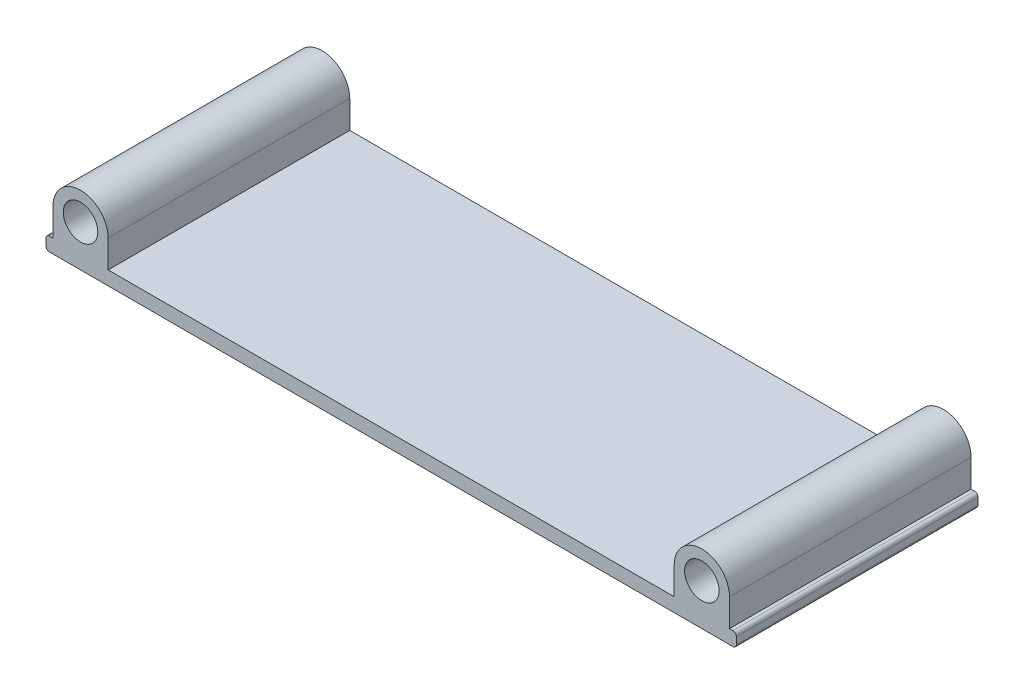
ISO-10303-21;
HEADER;
FILE_DESCRIPTION(('STEP AP214'),'2;1');
FILE_NAME('part.step','',(''),(''),'','','');
FILE_SCHEMA(('AUTOMOTIVE_DESIGN { 1 0 10303 214 1 1 1 1 }'));
ENDSEC;
DATA;
#1=APPLICATION_CONTEXT('core data for automotive mechanical design processes');
#2=APPLICATION_PROTOCOL_DEFINITION('international standard','automotive_design',2000,#1);
#3=PRODUCT_CONTEXT('',#1,'mechanical');
#4=PRODUCT('Part','Part','',(#3));
#5=PRODUCT_RELATED_PRODUCT_CATEGORY('part','',(#4));
#6=PRODUCT_DEFINITION_FORMATION('','',#4);
#7=PRODUCT_DEFINITION_CONTEXT('part definition',#1,'design');
#8=PRODUCT_DEFINITION('design','',#6,#7);
#9=PRODUCT_DEFINITION_SHAPE('','',#8);
#10=(LENGTH_UNIT() NAMED_UNIT(*) SI_UNIT(.MILLI.,.METRE.));
#11=(NAMED_UNIT(*) PLANE_ANGLE_UNIT() SI_UNIT($,.RADIAN.));
#12=(NAMED_UNIT(*) SI_UNIT($,.STERADIAN.) SOLID_ANGLE_UNIT());
#13=UNCERTAINTY_MEASURE_WITH_UNIT(LENGTH_MEASURE(1.E-05),#10,'distance_accuracy_value','');
#14=(GEOMETRIC_REPRESENTATION_CONTEXT(3) GLOBAL_UNCERTAINTY_ASSIGNED_CONTEXT((#13)) GLOBAL_UNIT_ASSIGNED_CONTEXT((#10,
#11,#12)) REPRESENTATION_CONTEXT('',''));
#15=CARTESIAN_POINT('',(0.,0.,0.));
#16=DIRECTION('',(0.,0.,1.));
#17=DIRECTION('',(1.,0.,0.));
#18=AXIS2_PLACEMENT_3D('',#15,#16,#17);
#19=CARTESIAN_POINT('',(49.,0.,17.5));
#20=DIRECTION('',(-1.,0.,0.));
#21=DIRECTION('',(0.,0.,1.));
#22=AXIS2_PLACEMENT_3D('',#19,#20,#21);
#23=PLANE('',#22);
#24=DIRECTION('',(0.,1.,0.));
#25=VECTOR('',#24,1.);
#26=CARTESIAN_POINT('',(49.,0.,-17.5));
#27=LINE('',#26,#25);
#28=CARTESIAN_POINT('',(49.,1.,-17.5));
#29=VERTEX_POINT('',#28);
#30=CARTESIAN_POINT('',(49.,5.,-17.5));
#31=VERTEX_POINT('',#30);
#32=EDGE_CURVE('E176',#29,#31,#27,.T.);
#33=ORIENTED_EDGE('',*,*,#32,.T.);
#34=DIRECTION('',(0.,0.,-1.));
#35=VECTOR('',#34,1.);
#36=CARTESIAN_POINT('',(49.,5.,17.5));
#37=LINE('',#36,#35);
#38=CARTESIAN_POINT('',(49.,5.,17.5));
#39=VERTEX_POINT('',#38);
#40=EDGE_CURVE('E161',#39,#31,#37,.T.);
#41=ORIENTED_EDGE('',*,*,#40,.F.);
#42=DIRECTION('',(0.,1.,0.));
#43=VECTOR('',#42,1.);
#44=CARTESIAN_POINT('',(49.,0.,17.5));
#45=LINE('',#44,#43);
#46=CARTESIAN_POINT('',(49.,1.,17.5));
#47=VERTEX_POINT('',#46);
#48=EDGE_CURVE('E170',#47,#39,#45,.T.);
#49=ORIENTED_EDGE('',*,*,#48,.F.);
#50=DIRECTION('',(0.,0.,-1.));
#51=VECTOR('',#50,1.);
#52=CARTESIAN_POINT('',(49.,1.,17.5));
#53=LINE('',#52,#51);
#54=EDGE_CURVE('E245',#47,#29,#53,.T.);
#55=ORIENTED_EDGE('',*,*,#54,.T.);
#56=EDGE_LOOP('',(#33,#41,#49,#55));
#57=FACE_BOUND('',#56,.T.);
#58=ADVANCED_FACE('F41',(#57),#23,.F.);
#59=CARTESIAN_POINT('',(45.,5.,17.5));
#60=DIRECTION('',(0.,0.,-1.));
#61=DIRECTION('',(-1.,0.,0.));
#62=AXIS2_PLACEMENT_3D('',#59,#60,#61);
#63=CYLINDRICAL_SURFACE('',#62,4.);
#64=CARTESIAN_POINT('',(45.,5.,-17.5));
#65=DIRECTION('',(0.,0.,1.));
#66=DIRECTION('',(1.,0.,0.));
#67=AXIS2_PLACEMENT_3D('',#64,#65,#66);
#68=CIRCLE('',#67,4.);
#69=CARTESIAN_POINT('',(41.,5.,-17.5));
#70=VERTEX_POINT('',#69);
#71=EDGE_CURVE('E267',#31,#70,#68,.T.);
#72=ORIENTED_EDGE('',*,*,#71,.T.);
#73=DIRECTION('',(0.,0.,-1.));
#74=VECTOR('',#73,1.);
#75=CARTESIAN_POINT('',(41.,5.,17.5));
#76=LINE('',#75,#74);
#77=CARTESIAN_POINT('',(41.,5.,17.5));
#78=VERTEX_POINT('',#77);
#79=EDGE_CURVE('E162',#78,#70,#76,.T.);
#80=ORIENTED_EDGE('',*,*,#79,.F.);
#81=CARTESIAN_POINT('',(45.,5.,17.5));
#82=DIRECTION('',(0.,0.,1.));
#83=DIRECTION('',(1.,0.,0.));
#84=AXIS2_PLACEMENT_3D('',#81,#82,#83);
#85=CIRCLE('',#84,4.);
#86=EDGE_CURVE('E156',#39,#78,#85,.T.);
#87=ORIENTED_EDGE('',*,*,#86,.F.);
#88=ORIENTED_EDGE('',*,*,#40,.T.);
#89=EDGE_LOOP('',(#72,#80,#87,#88));
#90=FACE_BOUND('',#89,.T.);
#91=ADVANCED_FACE('F157',(#90),#63,.T.);
#92=CARTESIAN_POINT('',(41.,0.,17.5));
#93=DIRECTION('',(-1.,0.,0.));
#94=DIRECTION('',(0.,0.,1.));
#95=AXIS2_PLACEMENT_3D('',#92,#93,#94);
#96=PLANE('',#95);
#97=DIRECTION('',(0.,1.,0.));
#98=VECTOR('',#97,1.);
#99=CARTESIAN_POINT('',(41.,0.,-17.5));
#100=LINE('',#99,#98);
#101=CARTESIAN_POINT('',(41.,1.,-17.5));
#102=VERTEX_POINT('',#101);
#103=EDGE_CURVE('E270',#102,#70,#100,.T.);
#104=ORIENTED_EDGE('',*,*,#103,.F.);
#105=DIRECTION('',(0.,0.,-1.));
#106=VECTOR('',#105,1.);
#107=CARTESIAN_POINT('',(41.,1.,17.5));
#108=LINE('',#107,#106);
#109=CARTESIAN_POINT('',(41.,1.,17.5));
#110=VERTEX_POINT('',#109);
#111=EDGE_CURVE('E181',#110,#102,#108,.T.);
#112=ORIENTED_EDGE('',*,*,#111,.F.);
#113=DIRECTION('',(0.,1.,0.));
#114=VECTOR('',#113,1.);
#115=CARTESIAN_POINT('',(41.,0.,17.5));
#116=LINE('',#115,#114);
#117=EDGE_CURVE('E167',#110,#78,#116,.T.);
#118=ORIENTED_EDGE('',*,*,#117,.T.);
#119=ORIENTED_EDGE('',*,*,#79,.T.);
#120=EDGE_LOOP('',(#104,#112,#118,#119));
#121=FACE_BOUND('',#120,.T.);
#122=ADVANCED_FACE('F268',(#121),#96,.T.);
#123=CARTESIAN_POINT('',(0.,1.,17.5));
#124=DIRECTION('',(0.,1.,0.));
#125=DIRECTION('',(0.,0.,1.));
#126=AXIS2_PLACEMENT_3D('',#123,#124,#125);
#127=PLANE('',#126);
#128=DIRECTION('',(1.,0.,0.));
#129=VECTOR('',#128,1.);
#130=CARTESIAN_POINT('',(0.,1.,-17.5));
#131=LINE('',#130,#129);
#132=CARTESIAN_POINT('',(-41.,1.,-17.5));
#133=VERTEX_POINT('',#132);
#134=EDGE_CURVE('E265',#133,#102,#131,.T.);
#135=ORIENTED_EDGE('',*,*,#134,.F.);
#136=DIRECTION('',(0.,0.,-1.));
#137=VECTOR('',#136,1.);
#138=CARTESIAN_POINT('',(-41.,1.,17.5));
#139=LINE('',#138,#137);
#140=CARTESIAN_POINT('',(-41.,1.,17.5));
#141=VERTEX_POINT('',#140);
#142=EDGE_CURVE('E254',#141,#133,#139,.T.);
#143=ORIENTED_EDGE('',*,*,#142,.F.);
#144=DIRECTION('',(1.,0.,0.));
#145=VECTOR('',#144,1.);
#146=CARTESIAN_POINT('',(0.,1.,17.5));
#147=LINE('',#146,#145);
#148=EDGE_CURVE('E262',#141,#110,#147,.T.);
#149=ORIENTED_EDGE('',*,*,#148,.T.);
#150=ORIENTED_EDGE('',*,*,#111,.T.);
#151=EDGE_LOOP('',(#135,#143,#149,#150));
#152=FACE_BOUND('',#151,.T.);
#153=ADVANCED_FACE('F257',(#152),#127,.T.);
#154=CARTESIAN_POINT('',(-41.,0.,17.5));
#155=DIRECTION('',(-1.,0.,0.));
#156=DIRECTION('',(0.,0.,1.));
#157=AXIS2_PLACEMENT_3D('',#154,#155,#156);
#158=PLANE('',#157);
#159=DIRECTION('',(0.,1.,0.));
#160=VECTOR('',#159,1.);
#161=CARTESIAN_POINT('',(-41.,0.,-17.5));
#162=LINE('',#161,#160);
#163=CARTESIAN_POINT('',(-41.,5.,-17.5));
#164=VERTEX_POINT('',#163);
#165=EDGE_CURVE('E272',#133,#164,#162,.T.);
#166=ORIENTED_EDGE('',*,*,#165,.T.);
#167=DIRECTION('',(0.,0.,-1.));
#168=VECTOR('',#167,1.);
#169=CARTESIAN_POINT('',(-41.,5.,17.5));
#170=LINE('',#169,#168);
#171=CARTESIAN_POINT('',(-41.,5.,17.5));
#172=VERTEX_POINT('',#171);
#173=EDGE_CURVE('E252',#172,#164,#170,.T.);
#174=ORIENTED_EDGE('',*,*,#173,.F.);
#175=DIRECTION('',(0.,1.,0.));
#176=VECTOR('',#175,1.);
#177=CARTESIAN_POINT('',(-41.,0.,17.5));
#178=LINE('',#177,#176);
#179=EDGE_CURVE('E299',#141,#172,#178,.T.);
#180=ORIENTED_EDGE('',*,*,#179,.F.);
#181=ORIENTED_EDGE('',*,*,#142,.T.);
#182=EDGE_LOOP('',(#166,#174,#180,#181));
#183=FACE_BOUND('',#182,.T.);
#184=ADVANCED_FACE('F298',(#183),#158,.F.);
#185=CARTESIAN_POINT('',(-45.,5.,17.5));
#186=DIRECTION('',(0.,0.,-1.));
#187=DIRECTION('',(-1.,0.,0.));
#188=AXIS2_PLACEMENT_3D('',#185,#186,#187);
#189=CYLINDRICAL_SURFACE('',#188,4.);
#190=CARTESIAN_POINT('',(-45.,5.,-17.5));
#191=DIRECTION('',(0.,0.,1.));
#192=DIRECTION('',(1.,0.,0.));
#193=AXIS2_PLACEMENT_3D('',#190,#191,#192);
#194=CIRCLE('',#193,4.);
#195=CARTESIAN_POINT('',(-49.,5.,-17.5));
#196=VERTEX_POINT('',#195);
#197=EDGE_CURVE('E274',#164,#196,#194,.T.);
#198=ORIENTED_EDGE('',*,*,#197,.T.);
#199=DIRECTION('',(0.,0.,-1.));
#200=VECTOR('',#199,1.);
#201=CARTESIAN_POINT('',(-49.,5.,17.5));
#202=LINE('',#201,#200);
#203=CARTESIAN_POINT('',(-49.,5.,17.5));
#204=VERTEX_POINT('',#203);
#205=EDGE_CURVE('E249',#204,#196,#202,.T.);
#206=ORIENTED_EDGE('',*,*,#205,.F.);
#207=CARTESIAN_POINT('',(-45.,5.,17.5));
#208=DIRECTION('',(0.,0.,1.));
#209=DIRECTION('',(1.,0.,0.));
#210=AXIS2_PLACEMENT_3D('',#207,#208,#209);
#211=CIRCLE('',#210,4.);
#212=EDGE_CURVE('E291',#172,#204,#211,.T.);
#213=ORIENTED_EDGE('',*,*,#212,.F.);
#214=ORIENTED_EDGE('',*,*,#173,.T.);
#215=EDGE_LOOP('',(#198,#206,#213,#214));
#216=FACE_BOUND('',#215,.T.);
#217=ADVANCED_FACE('F292',(#216),#189,.T.);
#218=CARTESIAN_POINT('',(-49.,0.,17.5));
#219=DIRECTION('',(-1.,0.,0.));
#220=DIRECTION('',(0.,0.,1.));
#221=AXIS2_PLACEMENT_3D('',#218,#219,#220);
#222=PLANE('',#221);
#223=DIRECTION('',(0.,1.,0.));
#224=VECTOR('',#223,1.);
#225=CARTESIAN_POINT('',(-49.,0.,-17.5));
#226=LINE('',#225,#224);
#227=CARTESIAN_POINT('',(-49.,1.,-17.5));
#228=VERTEX_POINT('',#227);
#229=EDGE_CURVE('E231',#228,#196,#226,.T.);
#230=ORIENTED_EDGE('',*,*,#229,.F.);
#231=DIRECTION('',(0.,0.,-1.));
#232=VECTOR('',#231,1.);
#233=CARTESIAN_POINT('',(-49.,1.,17.5));
#234=LINE('',#233,#232);
#235=CARTESIAN_POINT('',(-49.,1.,17.5));
#236=VERTEX_POINT('',#235);
#237=EDGE_CURVE('E248',#236,#228,#234,.T.);
#238=ORIENTED_EDGE('',*,*,#237,.F.);
#239=DIRECTION('',(0.,1.,0.));
#240=VECTOR('',#239,1.);
#241=CARTESIAN_POINT('',(-49.,0.,17.5));
#242=LINE('',#241,#240);
#243=EDGE_CURVE('E286',#236,#204,#242,.T.);
#244=ORIENTED_EDGE('',*,*,#243,.T.);
#245=ORIENTED_EDGE('',*,*,#205,.T.);
#246=EDGE_LOOP('',(#230,#238,#244,#245));
#247=FACE_BOUND('',#246,.T.);
#248=ADVANCED_FACE('F285',(#247),#222,.T.);
#249=CARTESIAN_POINT('',(0.,1.,17.5));
#250=DIRECTION('',(0.,1.,0.));
#251=DIRECTION('',(0.,0.,1.));
#252=AXIS2_PLACEMENT_3D('',#249,#250,#251);
#253=PLANE('',#252);
#254=DIRECTION('',(1.,0.,0.));
#255=VECTOR('',#254,1.);
#256=CARTESIAN_POINT('',(0.,1.,-17.5));
#257=LINE('',#256,#255);
#258=CARTESIAN_POINT('',(-49.5,1.,-17.5));
#259=VERTEX_POINT('',#258);
#260=EDGE_CURVE('E227',#259,#228,#257,.T.);
#261=ORIENTED_EDGE('',*,*,#260,.F.);
#262=DIRECTION('',(0.,0.,-1.));
#263=VECTOR('',#262,1.);
#264=CARTESIAN_POINT('',(-49.5,1.,17.5));
#265=LINE('',#264,#263);
#266=CARTESIAN_POINT('',(-49.5,1.,17.5));
#267=VERTEX_POINT('',#266);
#268=EDGE_CURVE('E11',#259,#267,#265,.F.);
#269=ORIENTED_EDGE('',*,*,#268,.T.);
#270=DIRECTION('',(1.,0.,0.));
#271=VECTOR('',#270,1.);
#272=CARTESIAN_POINT('',(0.,1.,17.5));
#273=LINE('',#272,#271);
#274=EDGE_CURVE('E302',#267,#236,#273,.T.);
#275=ORIENTED_EDGE('',*,*,#274,.T.);
#276=ORIENTED_EDGE('',*,*,#237,.T.);
#277=EDGE_LOOP('',(#261,#269,#275,#276));
#278=FACE_BOUND('',#277,.T.);
#279=ADVANCED_FACE('F341',(#278),#253,.T.);
#280=CARTESIAN_POINT('',(-50.,0.,17.5));
#281=DIRECTION('',(1.,0.,0.));
#282=DIRECTION('',(0.,0.,-1.));
#283=AXIS2_PLACEMENT_3D('',#280,#281,#282);
#284=PLANE('',#283);
#285=DIRECTION('',(0.,-1.,0.));
#286=VECTOR('',#285,1.);
#287=CARTESIAN_POINT('',(-50.,0.,-17.5));
#288=LINE('',#287,#286);
#289=CARTESIAN_POINT('',(-50.,0.5,-17.5));
#290=VERTEX_POINT('',#289);
#291=CARTESIAN_POINT('',(-50.,-0.5,-17.5));
#292=VERTEX_POINT('',#291);
#293=EDGE_CURVE('E220',#290,#292,#288,.T.);
#294=ORIENTED_EDGE('',*,*,#293,.T.);
#295=DIRECTION('',(0.,0.,-1.));
#296=VECTOR('',#295,1.);
#297=CARTESIAN_POINT('',(-50.,-0.5,17.5));
#298=LINE('',#297,#296);
#299=CARTESIAN_POINT('',(-50.,-0.5,17.5));
#300=VERTEX_POINT('',#299);
#301=EDGE_CURVE('E47',#292,#300,#298,.F.);
#302=ORIENTED_EDGE('',*,*,#301,.T.);
#303=DIRECTION('',(0.,-1.,0.));
#304=VECTOR('',#303,1.);
#305=CARTESIAN_POINT('',(-50.,0.,17.5));
#306=LINE('',#305,#304);
#307=CARTESIAN_POINT('',(-50.,0.5,17.5));
#308=VERTEX_POINT('',#307);
#309=EDGE_CURVE('E217',#308,#300,#306,.T.);
#310=ORIENTED_EDGE('',*,*,#309,.F.);
#311=DIRECTION('',(0.,0.,-1.));
#312=VECTOR('',#311,1.);
#313=CARTESIAN_POINT('',(-50.,0.5,-17.5));
#314=LINE('',#313,#312);
#315=EDGE_CURVE('E215',#308,#290,#314,.T.);
#316=ORIENTED_EDGE('',*,*,#315,.T.);
#317=EDGE_LOOP('',(#294,#302,#310,#316));
#318=FACE_BOUND('',#317,.T.);
#319=ADVANCED_FACE('F216',(#318),#284,.F.);
#320=CARTESIAN_POINT('',(0.,-1.,17.5));
#321=DIRECTION('',(0.,1.,0.));
#322=DIRECTION('',(0.,0.,1.));
#323=AXIS2_PLACEMENT_3D('',#320,#321,#322);
#324=PLANE('',#323);
#325=DIRECTION('',(1.,0.,0.));
#326=VECTOR('',#325,1.);
#327=CARTESIAN_POINT('',(0.,-1.,-17.5));
#328=LINE('',#327,#326);
#329=CARTESIAN_POINT('',(-49.5,-1.,-17.5));
#330=VERTEX_POINT('',#329);
#331=CARTESIAN_POINT('',(49.5,-1.,-17.5));
#332=VERTEX_POINT('',#331);
#333=EDGE_CURVE('E229',#330,#332,#328,.T.);
#334=ORIENTED_EDGE('',*,*,#333,.T.);
#335=DIRECTION('',(0.,0.,-1.));
#336=VECTOR('',#335,1.);
#337=CARTESIAN_POINT('',(49.5,-1.,17.5));
#338=LINE('',#337,#336);
#339=CARTESIAN_POINT('',(49.5,-1.,17.5));
#340=VERTEX_POINT('',#339);
#341=EDGE_CURVE('E199',#332,#340,#338,.F.);
#342=ORIENTED_EDGE('',*,*,#341,.T.);
#343=DIRECTION('',(1.,0.,0.));
#344=VECTOR('',#343,1.);
#345=CARTESIAN_POINT('',(0.,-1.,17.5));
#346=LINE('',#345,#344);
#347=CARTESIAN_POINT('',(-49.5,-1.,17.5));
#348=VERTEX_POINT('',#347);
#349=EDGE_CURVE('E307',#348,#340,#346,.T.);
#350=ORIENTED_EDGE('',*,*,#349,.F.);
#351=DIRECTION('',(0.,0.,-1.));
#352=VECTOR('',#351,1.);
#353=CARTESIAN_POINT('',(-49.5,-1.,17.5));
#354=LINE('',#353,#352);
#355=EDGE_CURVE('E197',#348,#330,#354,.T.);
#356=ORIENTED_EDGE('',*,*,#355,.T.);
#357=EDGE_LOOP('',(#334,#342,#350,#356));
#358=FACE_BOUND('',#357,.T.);
#359=ADVANCED_FACE('F331',(#358),#324,.F.);
#360=CARTESIAN_POINT('',(50.,0.,17.5));
#361=DIRECTION('',(1.,0.,0.));
#362=DIRECTION('',(0.,0.,-1.));
#363=AXIS2_PLACEMENT_3D('',#360,#361,#362);
#364=PLANE('',#363);
#365=DIRECTION('',(0.,-1.,0.));
#366=VECTOR('',#365,1.);
#367=CARTESIAN_POINT('',(50.,0.,17.5));
#368=LINE('',#367,#366);
#369=CARTESIAN_POINT('',(50.,0.5,17.5));
#370=VERTEX_POINT('',#369);
#371=CARTESIAN_POINT('',(50.,-0.5,17.5));
#372=VERTEX_POINT('',#371);
#373=EDGE_CURVE('E310',#370,#372,#368,.T.);
#374=ORIENTED_EDGE('',*,*,#373,.T.);
#375=DIRECTION('',(0.,0.,-1.));
#376=VECTOR('',#375,1.);
#377=CARTESIAN_POINT('',(50.,-0.5,-17.5));
#378=LINE('',#377,#376);
#379=CARTESIAN_POINT('',(50.,-0.5,-17.5));
#380=VERTEX_POINT('',#379);
#381=EDGE_CURVE('E182',#372,#380,#378,.T.);
#382=ORIENTED_EDGE('',*,*,#381,.T.);
#383=DIRECTION('',(0.,-1.,0.));
#384=VECTOR('',#383,1.);
#385=CARTESIAN_POINT('',(50.,0.,-17.5));
#386=LINE('',#385,#384);
#387=CARTESIAN_POINT('',(50.,0.5,-17.5));
#388=VERTEX_POINT('',#387);
#389=EDGE_CURVE('E233',#388,#380,#386,.T.);
#390=ORIENTED_EDGE('',*,*,#389,.F.);
#391=DIRECTION('',(0.,0.,-1.));
#392=VECTOR('',#391,1.);
#393=CARTESIAN_POINT('',(50.,0.5,17.5));
#394=LINE('',#393,#392);
#395=EDGE_CURVE('E177',#388,#370,#394,.F.);
#396=ORIENTED_EDGE('',*,*,#395,.T.);
#397=EDGE_LOOP('',(#374,#382,#390,#396));
#398=FACE_BOUND('',#397,.T.);
#399=ADVANCED_FACE('F330',(#398),#364,.T.);
#400=CARTESIAN_POINT('',(0.,1.,17.5));
#401=DIRECTION('',(0.,1.,0.));
#402=DIRECTION('',(0.,0.,1.));
#403=AXIS2_PLACEMENT_3D('',#400,#401,#402);
#404=PLANE('',#403);
#405=DIRECTION('',(1.,0.,0.));
#406=VECTOR('',#405,1.);
#407=CARTESIAN_POINT('',(0.,1.,17.5));
#408=LINE('',#407,#406);
#409=CARTESIAN_POINT('',(49.5,1.,17.5));
#410=VERTEX_POINT('',#409);
#411=EDGE_CURVE('E172',#47,#410,#408,.T.);
#412=ORIENTED_EDGE('',*,*,#411,.T.);
#413=DIRECTION('',(0.,0.,-1.));
#414=VECTOR('',#413,1.);
#415=CARTESIAN_POINT('',(49.5,1.,17.5));
#416=LINE('',#415,#414);
#417=CARTESIAN_POINT('',(49.5,1.,-17.5));
#418=VERTEX_POINT('',#417);
#419=EDGE_CURVE('E207',#410,#418,#416,.T.);
#420=ORIENTED_EDGE('',*,*,#419,.T.);
#421=DIRECTION('',(1.,0.,0.));
#422=VECTOR('',#421,1.);
#423=CARTESIAN_POINT('',(0.,1.,-17.5));
#424=LINE('',#423,#422);
#425=EDGE_CURVE('E236',#29,#418,#424,.T.);
#426=ORIENTED_EDGE('',*,*,#425,.F.);
#427=ORIENTED_EDGE('',*,*,#54,.F.);
#428=EDGE_LOOP('',(#412,#420,#426,#427));
#429=FACE_BOUND('',#428,.T.);
#430=ADVANCED_FACE('F319',(#429),#404,.T.);
#431=CARTESIAN_POINT('',(45.,5.,17.5));
#432=DIRECTION('',(0.,0.,-1.));
#433=DIRECTION('',(-1.,0.,0.));
#434=AXIS2_PLACEMENT_3D('',#431,#432,#433);
#435=CYLINDRICAL_SURFACE('',#434,2.5);
#436=CARTESIAN_POINT('',(45.,5.,17.5));
#437=DIRECTION('',(0.,0.,1.));
#438=DIRECTION('',(1.,0.,0.));
#439=AXIS2_PLACEMENT_3D('',#436,#437,#438);
#440=CIRCLE('',#439,2.5);
#441=CARTESIAN_POINT('',(47.5,5.,17.5));
#442=VERTEX_POINT('',#441);
#443=EDGE_CURVE('E171',#442,#442,#440,.T.);
#444=ORIENTED_EDGE('',*,*,#443,.T.);
#445=EDGE_LOOP('',(#444));
#446=FACE_BOUND('',#445,.T.);
#447=CARTESIAN_POINT('',(45.,5.,-17.5));
#448=DIRECTION('',(0.,0.,1.));
#449=DIRECTION('',(1.,0.,0.));
#450=AXIS2_PLACEMENT_3D('',#447,#448,#449);
#451=CIRCLE('',#450,2.5);
#452=CARTESIAN_POINT('',(47.5,5.,-17.5));
#453=VERTEX_POINT('',#452);
#454=EDGE_CURVE('E312',#453,#453,#451,.T.);
#455=ORIENTED_EDGE('',*,*,#454,.F.);
#456=EDGE_LOOP('',(#455));
#457=FACE_BOUND('',#456,.T.);
#458=ADVANCED_FACE('F363',(#446,#457),#435,.F.);
#459=CARTESIAN_POINT('',(-45.,5.,17.5));
#460=DIRECTION('',(0.,0.,-1.));
#461=DIRECTION('',(-1.,0.,0.));
#462=AXIS2_PLACEMENT_3D('',#459,#460,#461);
#463=CYLINDRICAL_SURFACE('',#462,2.5);
#464=CARTESIAN_POINT('',(-45.,5.,17.5));
#465=DIRECTION('',(0.,0.,1.));
#466=DIRECTION('',(1.,0.,0.));
#467=AXIS2_PLACEMENT_3D('',#464,#465,#466);
#468=CIRCLE('',#467,2.5);
#469=CARTESIAN_POINT('',(-42.5,5.,17.5));
#470=VERTEX_POINT('',#469);
#471=EDGE_CURVE('E250',#470,#470,#468,.T.);
#472=ORIENTED_EDGE('',*,*,#471,.T.);
#473=EDGE_LOOP('',(#472));
#474=FACE_BOUND('',#473,.T.);
#475=CARTESIAN_POINT('',(-45.,5.,-17.5));
#476=DIRECTION('',(0.,0.,1.));
#477=DIRECTION('',(1.,0.,0.));
#478=AXIS2_PLACEMENT_3D('',#475,#476,#477);
#479=CIRCLE('',#478,2.5);
#480=CARTESIAN_POINT('',(-42.5,5.,-17.5));
#481=VERTEX_POINT('',#480);
#482=EDGE_CURVE('E243',#481,#481,#479,.T.);
#483=ORIENTED_EDGE('',*,*,#482,.F.);
#484=EDGE_LOOP('',(#483));
#485=FACE_BOUND('',#484,.T.);
#486=ADVANCED_FACE('F365',(#474,#485),#463,.F.);
#487=CARTESIAN_POINT('',(0.,0.,17.5));
#488=DIRECTION('',(0.,0.,1.));
#489=DIRECTION('',(1.,0.,0.));
#490=AXIS2_PLACEMENT_3D('',#487,#488,#489);
#491=PLANE('',#490);
#492=ORIENTED_EDGE('',*,*,#443,.F.);
#493=EDGE_LOOP('',(#492));
#494=FACE_BOUND('',#493,.T.);
#495=ORIENTED_EDGE('',*,*,#349,.T.);
#496=CARTESIAN_POINT('',(49.5,-0.5,17.5));
#497=DIRECTION('',(0.,0.,1.));
#498=DIRECTION('',(1.,0.,0.));
#499=AXIS2_PLACEMENT_3D('',#496,#497,#498);
#500=CIRCLE('',#499,0.5);
#501=EDGE_CURVE('E210',#340,#372,#500,.T.);
#502=ORIENTED_EDGE('',*,*,#501,.T.);
#503=ORIENTED_EDGE('',*,*,#373,.F.);
#504=CARTESIAN_POINT('',(49.5,0.5,17.5));
#505=DIRECTION('',(0.,0.,1.));
#506=DIRECTION('',(1.,0.,0.));
#507=AXIS2_PLACEMENT_3D('',#504,#505,#506);
#508=CIRCLE('',#507,0.5);
#509=EDGE_CURVE('E57',#370,#410,#508,.T.);
#510=ORIENTED_EDGE('',*,*,#509,.T.);
#511=ORIENTED_EDGE('',*,*,#411,.F.);
#512=ORIENTED_EDGE('',*,*,#48,.T.);
#513=ORIENTED_EDGE('',*,*,#86,.T.);
#514=ORIENTED_EDGE('',*,*,#117,.F.);
#515=ORIENTED_EDGE('',*,*,#148,.F.);
#516=ORIENTED_EDGE('',*,*,#179,.T.);
#517=ORIENTED_EDGE('',*,*,#212,.T.);
#518=ORIENTED_EDGE('',*,*,#243,.F.);
#519=ORIENTED_EDGE('',*,*,#274,.F.);
#520=CARTESIAN_POINT('',(-49.5,0.5,17.5));
#521=DIRECTION('',(0.,0.,1.));
#522=DIRECTION('',(1.,0.,0.));
#523=AXIS2_PLACEMENT_3D('',#520,#521,#522);
#524=CIRCLE('',#523,0.5);
#525=EDGE_CURVE('E205',#267,#308,#524,.T.);
#526=ORIENTED_EDGE('',*,*,#525,.T.);
#527=ORIENTED_EDGE('',*,*,#309,.T.);
#528=CARTESIAN_POINT('',(-49.5,-0.5,17.5));
#529=DIRECTION('',(0.,0.,1.));
#530=DIRECTION('',(1.,0.,0.));
#531=AXIS2_PLACEMENT_3D('',#528,#529,#530);
#532=CIRCLE('',#531,0.5);
#533=EDGE_CURVE('E204',#300,#348,#532,.T.);
#534=ORIENTED_EDGE('',*,*,#533,.T.);
#535=EDGE_LOOP('',(#495,#502,#503,#510,#511,#512,#513,#514,#515,#516,#517,#518,#519,#526,#527,#534));
#536=FACE_BOUND('',#535,.T.);
#537=ORIENTED_EDGE('',*,*,#471,.F.);
#538=EDGE_LOOP('',(#537));
#539=FACE_BOUND('',#538,.T.);
#540=ADVANCED_FACE('F173',(#494,#536,#539),#491,.T.);
#541=CARTESIAN_POINT('',(0.,0.,-17.5));
#542=DIRECTION('',(0.,0.,1.));
#543=DIRECTION('',(1.,0.,0.));
#544=AXIS2_PLACEMENT_3D('',#541,#542,#543);
#545=PLANE('',#544);
#546=ORIENTED_EDGE('',*,*,#454,.T.);
#547=EDGE_LOOP('',(#546));
#548=FACE_BOUND('',#547,.T.);
#549=ORIENTED_EDGE('',*,*,#389,.T.);
#550=CARTESIAN_POINT('',(49.5,-0.5,-17.5));
#551=DIRECTION('',(0.,0.,1.));
#552=DIRECTION('',(1.,0.,0.));
#553=AXIS2_PLACEMENT_3D('',#550,#551,#552);
#554=CIRCLE('',#553,0.5);
#555=EDGE_CURVE('E194',#380,#332,#554,.F.);
#556=ORIENTED_EDGE('',*,*,#555,.T.);
#557=ORIENTED_EDGE('',*,*,#333,.F.);
#558=CARTESIAN_POINT('',(-49.5,-0.5,-17.5));
#559=DIRECTION('',(0.,0.,1.));
#560=DIRECTION('',(1.,0.,0.));
#561=AXIS2_PLACEMENT_3D('',#558,#559,#560);
#562=CIRCLE('',#561,0.5);
#563=EDGE_CURVE('E193',#330,#292,#562,.F.);
#564=ORIENTED_EDGE('',*,*,#563,.T.);
#565=ORIENTED_EDGE('',*,*,#293,.F.);
#566=CARTESIAN_POINT('',(-49.5,0.5,-17.5));
#567=DIRECTION('',(0.,0.,1.));
#568=DIRECTION('',(1.,0.,0.));
#569=AXIS2_PLACEMENT_3D('',#566,#567,#568);
#570=CIRCLE('',#569,0.5);
#571=EDGE_CURVE('E190',#290,#259,#570,.F.);
#572=ORIENTED_EDGE('',*,*,#571,.T.);
#573=ORIENTED_EDGE('',*,*,#260,.T.);
#574=ORIENTED_EDGE('',*,*,#229,.T.);
#575=ORIENTED_EDGE('',*,*,#197,.F.);
#576=ORIENTED_EDGE('',*,*,#165,.F.);
#577=ORIENTED_EDGE('',*,*,#134,.T.);
#578=ORIENTED_EDGE('',*,*,#103,.T.);
#579=ORIENTED_EDGE('',*,*,#71,.F.);
#580=ORIENTED_EDGE('',*,*,#32,.F.);
#581=ORIENTED_EDGE('',*,*,#425,.T.);
#582=CARTESIAN_POINT('',(49.5,0.5,-17.5));
#583=DIRECTION('',(0.,0.,1.));
#584=DIRECTION('',(1.,0.,0.));
#585=AXIS2_PLACEMENT_3D('',#582,#583,#584);
#586=CIRCLE('',#585,0.5);
#587=EDGE_CURVE('E191',#418,#388,#586,.F.);
#588=ORIENTED_EDGE('',*,*,#587,.T.);
#589=EDGE_LOOP('',(#549,#556,#557,#564,#565,#572,#573,#574,#575,#576,#577,#578,#579,#580,#581,#588));
#590=FACE_BOUND('',#589,.T.);
#591=ORIENTED_EDGE('',*,*,#482,.T.);
#592=EDGE_LOOP('',(#591));
#593=FACE_BOUND('',#592,.T.);
#594=ADVANCED_FACE('F224',(#548,#590,#593),#545,.F.);
#595=CARTESIAN_POINT('',(49.5,-0.5,17.5));
#596=DIRECTION('',(0.,0.,1.));
#597=DIRECTION('',(1.,0.,0.));
#598=AXIS2_PLACEMENT_3D('',#595,#596,#597);
#599=CYLINDRICAL_SURFACE('',#598,0.5);
#600=ORIENTED_EDGE('',*,*,#501,.F.);
#601=ORIENTED_EDGE('',*,*,#341,.F.);
#602=ORIENTED_EDGE('',*,*,#555,.F.);
#603=ORIENTED_EDGE('',*,*,#381,.F.);
#604=EDGE_LOOP('',(#600,#601,#602,#603));
#605=FACE_BOUND('',#604,.T.);
#606=ADVANCED_FACE('F332',(#605),#599,.T.);
#607=CARTESIAN_POINT('',(49.5,0.5,17.5));
#608=DIRECTION('',(0.,0.,-1.));
#609=DIRECTION('',(-1.,0.,0.));
#610=AXIS2_PLACEMENT_3D('',#607,#608,#609);
#611=CYLINDRICAL_SURFACE('',#610,0.5);
#612=ORIENTED_EDGE('',*,*,#509,.F.);
#613=ORIENTED_EDGE('',*,*,#395,.F.);
#614=ORIENTED_EDGE('',*,*,#587,.F.);
#615=ORIENTED_EDGE('',*,*,#419,.F.);
#616=EDGE_LOOP('',(#612,#613,#614,#615));
#617=FACE_BOUND('',#616,.T.);
#618=ADVANCED_FACE('F323',(#617),#611,.T.);
#619=CARTESIAN_POINT('',(-49.5,-0.5,17.5));
#620=DIRECTION('',(0.,0.,-1.));
#621=DIRECTION('',(-1.,0.,0.));
#622=AXIS2_PLACEMENT_3D('',#619,#620,#621);
#623=CYLINDRICAL_SURFACE('',#622,0.5);
#624=ORIENTED_EDGE('',*,*,#533,.F.);
#625=ORIENTED_EDGE('',*,*,#301,.F.);
#626=ORIENTED_EDGE('',*,*,#563,.F.);
#627=ORIENTED_EDGE('',*,*,#355,.F.);
#628=EDGE_LOOP('',(#624,#625,#626,#627));
#629=FACE_BOUND('',#628,.T.);
#630=ADVANCED_FACE('F340',(#629),#623,.T.);
#631=CARTESIAN_POINT('',(-49.5,0.5,17.5));
#632=DIRECTION('',(0.,0.,1.));
#633=DIRECTION('',(1.,0.,0.));
#634=AXIS2_PLACEMENT_3D('',#631,#632,#633);
#635=CYLINDRICAL_SURFACE('',#634,0.5);
#636=ORIENTED_EDGE('',*,*,#525,.F.);
#637=ORIENTED_EDGE('',*,*,#268,.F.);
#638=ORIENTED_EDGE('',*,*,#571,.F.);
#639=ORIENTED_EDGE('',*,*,#315,.F.);
#640=EDGE_LOOP('',(#636,#637,#638,#639));
#641=FACE_BOUND('',#640,.T.);
#642=ADVANCED_FACE('F43',(#641),#635,.T.);
#643=CLOSED_SHELL('',(#58,#91,#122,#153,#184,#217,#248,#279,#319,#359,#399,#430,#458,#486,#540,
#594,#606,#618,#630,#642));
#644=MANIFOLD_SOLID_BREP('B2',#643);
#645=ADVANCED_BREP_SHAPE_REPRESENTATION('',(#18,#644),#14);
#646=SHAPE_DEFINITION_REPRESENTATION(#9,#645);
ENDSEC;
END-ISO-10303-21;
